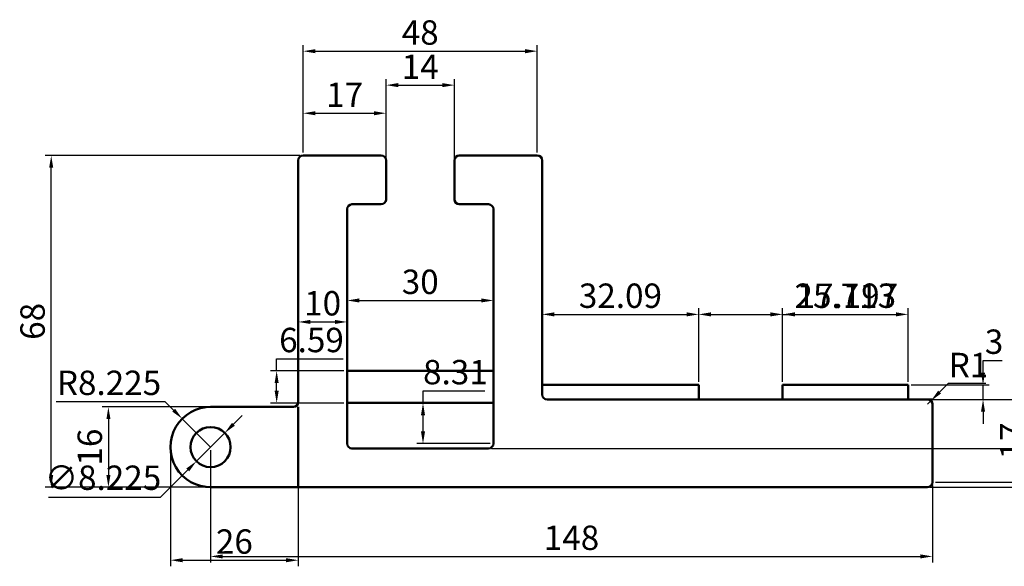
# Model space of a CAD drawing. Units: millimetres. Extents: x 2010 to 2347, y 1200 to 1429.
# Tile 2 of 3: x 2010 to 2212, y 1317 to 1429. Entities that reach past the tile are written whole.
import ezdxf

# ---------------------------------------------------------------- set-up
doc = ezdxf.new("R2010")
doc.units = ezdxf.units.MM
doc.layers.add('M-DIMS', color=2, linetype='Continuous', lineweight=25)
doc.layers.add('M-OUTL', color=7, linetype='Continuous', lineweight=50)
doc.styles.get("Standard").update_dxf_attribs({"font": 'arial.ttf'})
doc.dimstyles.new('ISO-25', dxfattribs={"dimtxt": 5, "dimasz": 2.5, "dimexe": 1.25, "dimexo": 0.625, "dimtad": 1, "dimtoh": 1, "dimdec": 0, "dimtxsty": 'Standard', "dimcen": 2.5, "dimadec": 0, "dimazin": 0, "dimtfac": 1, "dimtdec": 0, "dimtmove": 0, "dimatfit": 3, "dimfxl": 1, "dimarcsym": 0})

# ---------------------------------------------------------------- blocks, each defined once
blk = doc.blocks.new('*D1')
at = {"layer": 'Defpoints', "color": 0, "transparency": 16777216}
for p in [(2049.6, 1341.27), (2197.57, 1334.05), (2197.57, 1318.86)]:
    blk.add_point(p, dxfattribs=at)
at = {"layer": 'M-DIMS', "color": 0, "lineweight": -2, "transparency": 16777216}
for p, q in [((2049.6, 1340.65), (2049.6, 1317.61)), ((2197.57, 1333.42), (2197.57, 1317.61)), ((2052.1, 1318.86), (2195.07, 1318.86))]:
    blk.add_line(p, q, dxfattribs=at)
at = {"layer": 'M-DIMS', "color": 0, "transparency": 16777216}
for points in [[(2052.1, 1319.27), (2052.1, 1318.44), (2049.6, 1318.86)], [(2195.07, 1319.27), (2195.07, 1318.44), (2197.57, 1318.86)]]:
    blk.add_solid(points, dxfattribs=at)
at = {"layer": 'M-DIMS', "color": 0, "transparency": 16777216, "insert": (2123.58, 1322.03), "char_height": 5, "attachment_point": 5}
blk.add_mtext('148', dxfattribs=at)
blk = doc.blocks.new('*D2')
at = {"layer": 'Defpoints', "color": 0, "transparency": 16777216}
for p in [(2196.57, 1351.05), (2217.71, 1351.05), (2197.57, 1334.05)]:
    blk.add_point(p, dxfattribs=at)
at = {"layer": 'M-DIMS', "color": 0, "lineweight": -2, "transparency": 16777216}
for p, q in [((2197.19, 1351.05), (2218.96, 1351.05)), ((2217.71, 1336.55), (2217.71, 1348.55)), ((2198.19, 1334.05), (2218.96, 1334.05))]:
    blk.add_line(p, q, dxfattribs=at)
at = {"layer": 'M-DIMS', "color": 0, "transparency": 16777216}
for points in [[(2217.3, 1348.55), (2218.13, 1348.55), (2217.71, 1351.05)], [(2217.3, 1336.55), (2218.13, 1336.55), (2217.71, 1334.05)]]:
    blk.add_solid(points, dxfattribs=at)
at = {"layer": 'M-DIMS', "color": 0, "transparency": 16777216, "insert": (2214.58, 1342.55), "char_height": 5, "attachment_point": 5, "rotation": 90}
blk.add_mtext('17', dxfattribs=at)
blk = doc.blocks.new('*D3')
at = {"layer": 'Defpoints', "color": 0, "transparency": 16777216}
for p in [(2192.57, 1354.05), (2207.94, 1354.05), (2196.57, 1351.05)]:
    blk.add_point(p, dxfattribs=at)
at = {"layer": 'M-DIMS', "color": 0, "lineweight": -2, "transparency": 16777216}
for p, q in [((2207.94, 1356.55), (2207.94, 1359.05)), ((2207.94, 1359.05), (2211.84, 1359.05)), ((2193.19, 1354.05), (2209.19, 1354.05)), ((2207.94, 1351.05), (2207.94, 1354.05)), ((2197.19, 1351.05), (2209.19, 1351.05)), ((2207.94, 1348.55), (2207.94, 1346.05))]:
    blk.add_line(p, q, dxfattribs=at)
at = {"layer": 'M-DIMS', "color": 0, "transparency": 16777216}
for points in [[(2207.52, 1356.55), (2208.35, 1356.55), (2207.94, 1354.05)], [(2207.52, 1348.55), (2208.35, 1348.55), (2207.94, 1351.05)]]:
    blk.add_solid(points, dxfattribs=at)
at = {"layer": 'M-DIMS', "color": 0, "transparency": 16777216, "insert": (2210.2, 1362.23), "char_height": 5, "attachment_point": 5}
blk.add_mtext('3', dxfattribs=at)
blk = doc.blocks.new('*D4')
at = {"layer": 'Defpoints', "color": 0, "transparency": 16777216}
for p in [(2041.37, 1341.27), (2067.57, 1341.27), (2067.57, 1318.08)]:
    blk.add_point(p, dxfattribs=at)
at = {"layer": 'M-DIMS', "color": 0, "lineweight": -2, "transparency": 16777216}
for p, q in [((2041.37, 1340.65), (2041.37, 1316.83)), ((2067.57, 1340.65), (2067.57, 1316.83)), ((2043.87, 1318.08), (2065.07, 1318.08))]:
    blk.add_line(p, q, dxfattribs=at)
at = {"layer": 'M-DIMS', "color": 0, "transparency": 16777216}
for points in [[(2043.87, 1318.5), (2043.87, 1317.66), (2041.37, 1318.08)], [(2065.07, 1318.5), (2065.07, 1317.66), (2067.57, 1318.08)]]:
    blk.add_solid(points, dxfattribs=at)
at = {"layer": 'M-DIMS', "color": 0, "transparency": 16777216, "insert": (2054.47, 1321.26), "char_height": 5, "attachment_point": 5}
blk.add_mtext('26', dxfattribs=at)
blk = doc.blocks.new('*D5')
at = {"layer": 'Defpoints', "color": 0, "transparency": 16777216}
for p in [(2049.6, 1349.5), (2028.65, 1333.05), (2049.62, 1333.05)]:
    blk.add_point(p, dxfattribs=at)
at = {"layer": 'M-DIMS', "color": 0, "lineweight": -2, "transparency": 16777216}
for p, q in [((2048.97, 1349.5), (2027.4, 1349.5)), ((2028.65, 1347), (2028.65, 1335.55)), ((2049, 1333.05), (2027.4, 1333.05))]:
    blk.add_line(p, q, dxfattribs=at)
at = {"layer": 'M-DIMS', "color": 0, "transparency": 16777216}
for points in [[(2028.24, 1347), (2029.07, 1347), (2028.65, 1349.5)], [(2028.24, 1335.55), (2029.07, 1335.55), (2028.65, 1333.05)]]:
    blk.add_solid(points, dxfattribs=at)
at = {"layer": 'M-DIMS', "color": 0, "transparency": 16777216, "insert": (2025.48, 1341.27), "char_height": 5, "attachment_point": 5, "rotation": 90}
blk.add_mtext('16', dxfattribs=at)
blk = doc.blocks.new('*D6')
at = {"layer": 'Defpoints', "color": 0, "transparency": 16777216}
for p in [(2067.57, 1375.27), (2077.57, 1366.93), (2077.57, 1366.03)]:
    blk.add_point(p, dxfattribs=at)
at = {"layer": 'M-DIMS', "color": 0, "lineweight": -2, "transparency": 16777216}
for p, q in [((2067.57, 1374.65), (2067.57, 1365.68)), ((2070.07, 1366.93), (2075.07, 1366.93)), ((2077.57, 1366.65), (2077.57, 1368.18))]:
    blk.add_line(p, q, dxfattribs=at)
at = {"layer": 'M-DIMS', "color": 0, "transparency": 16777216}
for points in [[(2070.07, 1367.35), (2070.07, 1366.51), (2067.57, 1366.93)], [(2075.07, 1367.35), (2075.07, 1366.51), (2077.57, 1366.93)]]:
    blk.add_solid(points, dxfattribs=at)
at = {"layer": 'M-DIMS', "color": 0, "transparency": 16777216, "insert": (2072.57, 1370.11), "char_height": 5, "attachment_point": 5}
blk.add_mtext('10', dxfattribs=at)
blk = doc.blocks.new('*D7')
at = {"layer": 'Defpoints', "color": 0, "transparency": 16777216}
for p in [(2085.57, 1409.72), (2068.57, 1401.05), (2085.57, 1400.05)]:
    blk.add_point(p, dxfattribs=at)
at = {"layer": 'M-DIMS', "color": 0, "lineweight": -2, "transparency": 16777216}
for p, q in [((2068.57, 1401.67), (2068.57, 1410.97)), ((2085.57, 1400.67), (2085.57, 1410.97)), ((2071.07, 1409.72), (2083.07, 1409.72))]:
    blk.add_line(p, q, dxfattribs=at)
at = {"layer": 'M-DIMS', "color": 0, "transparency": 16777216}
for points in [[(2071.07, 1410.13), (2071.07, 1409.3), (2068.57, 1409.72)], [(2083.07, 1410.13), (2083.07, 1409.3), (2085.57, 1409.72)]]:
    blk.add_solid(points, dxfattribs=at)
at = {"layer": 'M-DIMS', "color": 0, "transparency": 16777216, "insert": (2077.07, 1412.85), "char_height": 5, "attachment_point": 5}
blk.add_mtext('17', dxfattribs=at)
blk = doc.blocks.new('*D8')
at = {"layer": 'Defpoints', "color": 0, "transparency": 16777216}
for p in [(2116.57, 1422.44), (2068.57, 1401.05), (2116.57, 1401.05)]:
    blk.add_point(p, dxfattribs=at)
at = {"layer": 'M-DIMS', "color": 0, "lineweight": -2, "transparency": 16777216}
for p, q in [((2068.57, 1401.67), (2068.57, 1423.69)), ((2116.57, 1401.67), (2116.57, 1423.69)), ((2071.07, 1422.44), (2114.07, 1422.44))]:
    blk.add_line(p, q, dxfattribs=at)
at = {"layer": 'M-DIMS', "color": 0, "transparency": 16777216}
for points in [[(2071.07, 1422.86), (2071.07, 1422.02), (2068.57, 1422.44)], [(2114.07, 1422.86), (2114.07, 1422.02), (2116.57, 1422.44)]]:
    blk.add_solid(points, dxfattribs=at)
at = {"layer": 'M-DIMS', "color": 0, "transparency": 16777216, "insert": (2092.57, 1425.62), "char_height": 5, "attachment_point": 5}
blk.add_mtext('48', dxfattribs=at)
blk = doc.blocks.new('*D25')
at = {"layer": 'Defpoints', "color": 0, "transparency": 16777216}
for p in [(2016.93, 1401.05), (2068.57, 1401.05), (2049.62, 1333.05)]:
    blk.add_point(p, dxfattribs=at)
at = {"layer": 'M-DIMS', "color": 0, "lineweight": -2, "transparency": 16777216}
for p, q in [((2067.94, 1401.05), (2015.68, 1401.05)), ((2016.93, 1335.55), (2016.93, 1398.55)), ((2049, 1333.05), (2015.68, 1333.05))]:
    blk.add_line(p, q, dxfattribs=at)
at = {"layer": 'M-DIMS', "color": 0, "transparency": 16777216}
for points in [[(2016.51, 1398.55), (2017.34, 1398.55), (2016.93, 1401.05)], [(2016.51, 1335.55), (2017.34, 1335.55), (2016.93, 1333.05)]]:
    blk.add_solid(points, dxfattribs=at)
at = {"layer": 'M-DIMS', "color": 0, "transparency": 16777216, "insert": (2013.75, 1367.05), "char_height": 5, "attachment_point": 5, "rotation": 90}
blk.add_mtext('68', dxfattribs=at)
blk = doc.blocks.new('*D32')
at = {"layer": 'Defpoints', "color": 0, "transparency": 16777216}
for p in [(2099.57, 1415.48), (2085.57, 1400.05), (2099.57, 1400.05)]:
    blk.add_point(p, dxfattribs=at)
at = {"layer": 'M-DIMS', "color": 0, "lineweight": -2, "transparency": 16777216}
for p, q in [((2085.57, 1400.67), (2085.57, 1416.73)), ((2088.07, 1415.48), (2097.07, 1415.48)), ((2099.57, 1400.67), (2099.57, 1416.73))]:
    blk.add_line(p, q, dxfattribs=at)
at = {"layer": 'M-DIMS', "color": 0, "transparency": 16777216}
for points in [[(2088.07, 1415.9), (2088.07, 1415.06), (2085.57, 1415.48)], [(2097.07, 1415.9), (2097.07, 1415.06), (2099.57, 1415.48)]]:
    blk.add_solid(points, dxfattribs=at)
at = {"layer": 'M-DIMS', "color": 0, "transparency": 16777216, "insert": (2092.57, 1418.61), "char_height": 5, "attachment_point": 5}
blk.add_mtext('14', dxfattribs=at)
blk = doc.blocks.new('*D36')
at = {"layer": 'Defpoints', "color": 0, "transparency": 16777216}
for p in [(2106.57, 1341), (2329.76, 1341), (2196.57, 1333.05)]:
    blk.add_point(p, dxfattribs=at)
at = {"layer": 'M-DIMS', "color": 0, "lineweight": -2, "transparency": 16777216}
for p, q in [((2329.76, 1341), (2329.76, 1343.5)), ((2329.76, 1343.5), (2347.26, 1343.5)), ((2107.19, 1341), (2331.01, 1341)), ((2329.76, 1335.55), (2329.76, 1338.5)), ((2197.19, 1333.05), (2331.01, 1333.05))]:
    blk.add_line(p, q, dxfattribs=at)
at = {"layer": 'M-DIMS', "color": 0, "transparency": 16777216}
for points in [[(2329.35, 1338.5), (2330.18, 1338.5), (2329.76, 1341)], [(2329.35, 1335.55), (2330.18, 1335.55), (2329.76, 1333.05)]]:
    blk.add_solid(points, dxfattribs=at)
at = {"layer": 'M-DIMS', "color": 0, "transparency": 16777216, "insert": (2338.82, 1346.68), "char_height": 5, "attachment_point": 5}
blk.add_mtext('7.955', dxfattribs=at)
blk = doc.blocks.new('*D37')
at = {"layer": 'Defpoints', "color": 0, "transparency": 16777216}
for p in [(2063.14, 1356.9), (2077.57, 1356.9), (2077.57, 1350.31)]:
    blk.add_point(p, dxfattribs=at)
at = {"layer": 'M-DIMS', "color": 0, "lineweight": -2, "transparency": 16777216}
for p, q in [((2063.14, 1356.9), (2063.14, 1359.4)), ((2063.14, 1359.4), (2076.79, 1359.4)), ((2076.94, 1356.9), (2061.89, 1356.9)), ((2063.14, 1352.81), (2063.14, 1354.4)), ((2076.94, 1350.31), (2061.89, 1350.31))]:
    blk.add_line(p, q, dxfattribs=at)
at = {"layer": 'M-DIMS', "color": 0, "transparency": 16777216}
for points in [[(2062.72, 1354.4), (2063.56, 1354.4), (2063.14, 1356.9)], [(2062.72, 1352.81), (2063.56, 1352.81), (2063.14, 1350.31)]]:
    blk.add_solid(points, dxfattribs=at)
at = {"layer": 'M-DIMS', "color": 0, "transparency": 16777216, "insert": (2070.28, 1362.58), "char_height": 5, "attachment_point": 5}
blk.add_mtext('6.59', dxfattribs=at)
blk = doc.blocks.new('*D38')
at = {"layer": 'Defpoints', "color": 0, "transparency": 16777216}
for p in [(2149.66, 1368.48), (2117.57, 1354.05), (2149.66, 1354.05)]:
    blk.add_point(p, dxfattribs=at)
at = {"layer": 'M-DIMS', "color": 0, "lineweight": -2, "transparency": 16777216}
for p, q in [((2117.57, 1354.67), (2117.57, 1369.73)), ((2120.07, 1368.48), (2147.16, 1368.48)), ((2149.66, 1354.67), (2149.66, 1369.73))]:
    blk.add_line(p, q, dxfattribs=at)
at = {"layer": 'M-DIMS', "color": 0, "transparency": 16777216}
for points in [[(2120.07, 1368.9), (2120.07, 1368.06), (2117.57, 1368.48)], [(2147.16, 1368.9), (2147.16, 1368.06), (2149.66, 1368.48)]]:
    blk.add_solid(points, dxfattribs=at)
at = {"layer": 'M-DIMS', "color": 0, "transparency": 16777216, "insert": (2133.61, 1371.66), "char_height": 5, "attachment_point": 5}
blk.add_mtext('32.09', dxfattribs=at)
blk = doc.blocks.new('*D39')
at = {"layer": 'Defpoints', "color": 0, "transparency": 16777216}
for p in [(2166.86, 1368.48), (2149.66, 1354.05), (2166.86, 1354.05)]:
    blk.add_point(p, dxfattribs=at)
at = {"layer": 'M-DIMS', "color": 0, "lineweight": -2, "transparency": 16777216}
for p, q in [((2149.66, 1354.67), (2149.66, 1369.73)), ((2152.16, 1368.48), (2164.36, 1368.48)), ((2166.86, 1354.67), (2166.86, 1369.73)), ((2166.86, 1368.48), (2190.89, 1368.48))]:
    blk.add_line(p, q, dxfattribs=at)
at = {"layer": 'M-DIMS', "color": 0, "transparency": 16777216}
for points in [[(2152.16, 1368.9), (2152.16, 1368.06), (2149.66, 1368.48)], [(2164.36, 1368.9), (2164.36, 1368.06), (2166.86, 1368.48)]]:
    blk.add_solid(points, dxfattribs=at)
at = {"layer": 'M-DIMS', "color": 0, "transparency": 16777216, "insert": (2180.12, 1371.66), "char_height": 5, "attachment_point": 5}
blk.add_mtext('17.197', dxfattribs=at)
blk = doc.blocks.new('*D40')
at = {"layer": 'Defpoints', "color": 0, "transparency": 16777216}
for p in [(2192.57, 1368.48), (2166.86, 1354.05), (2192.57, 1354.05)]:
    blk.add_point(p, dxfattribs=at)
at = {"layer": 'M-DIMS', "color": 0, "lineweight": -2, "transparency": 16777216}
for p, q in [((2166.86, 1354.67), (2166.86, 1369.73)), ((2169.36, 1368.48), (2190.07, 1368.48)), ((2192.57, 1354.67), (2192.57, 1369.73))]:
    blk.add_line(p, q, dxfattribs=at)
at = {"layer": 'M-DIMS', "color": 0, "transparency": 16777216}
for points in [[(2169.36, 1368.9), (2169.36, 1368.06), (2166.86, 1368.48)], [(2190.07, 1368.9), (2190.07, 1368.06), (2192.57, 1368.48)]]:
    blk.add_solid(points, dxfattribs=at)
at = {"layer": 'M-DIMS', "color": 0, "transparency": 16777216, "insert": (2179.71, 1371.66), "char_height": 5, "attachment_point": 5}
blk.add_mtext('25.713', dxfattribs=at)
blk = doc.blocks.new('*D41')
at = {"layer": 'Defpoints', "color": 0, "transparency": 16777216}
for p in [(2093.14, 1350.31), (2107.57, 1350.31), (2107.57, 1342)]:
    blk.add_point(p, dxfattribs=at)
at = {"layer": 'M-DIMS', "color": 0, "lineweight": -2, "transparency": 16777216}
for p, q in [((2093.14, 1350.31), (2093.14, 1352.81)), ((2093.14, 1352.81), (2105.79, 1352.81)), ((2106.94, 1350.31), (2091.89, 1350.31)), ((2093.14, 1344.5), (2093.14, 1347.81)), ((2106.94, 1342), (2091.89, 1342))]:
    blk.add_line(p, q, dxfattribs=at)
at = {"layer": 'M-DIMS', "color": 0, "transparency": 16777216}
for points in [[(2092.72, 1347.81), (2093.56, 1347.81), (2093.14, 1350.31)], [(2092.72, 1344.5), (2093.56, 1344.5), (2093.14, 1342)]]:
    blk.add_solid(points, dxfattribs=at)
at = {"layer": 'M-DIMS', "color": 0, "transparency": 16777216, "insert": (2099.78, 1355.99), "char_height": 5, "attachment_point": 5}
blk.add_mtext('8.31', dxfattribs=at)
blk = doc.blocks.new('*D44')
at = {"layer": 'Defpoints', "color": 0, "transparency": 16777216}
for p in [(2107.57, 1371.33), (2077.57, 1356.9), (2107.57, 1356.9)]:
    blk.add_point(p, dxfattribs=at)
at = {"layer": 'M-DIMS', "color": 0, "lineweight": -2, "transparency": 16777216}
for p, q in [((2077.57, 1357.53), (2077.57, 1372.58)), ((2107.57, 1357.53), (2107.57, 1372.58)), ((2080.07, 1371.33), (2105.07, 1371.33))]:
    blk.add_line(p, q, dxfattribs=at)
at = {"layer": 'M-DIMS', "color": 0, "transparency": 16777216}
for points in [[(2080.07, 1371.75), (2080.07, 1370.92), (2077.57, 1371.33)], [(2105.07, 1371.75), (2105.07, 1370.92), (2107.57, 1371.33)]]:
    blk.add_solid(points, dxfattribs=at)
at = {"layer": 'M-DIMS', "color": 0, "transparency": 16777216, "insert": (2092.57, 1374.51), "char_height": 5, "attachment_point": 5}
blk.add_mtext('30', dxfattribs=at)
blk = doc.blocks.new('*D51')
at = {"layer": 'Defpoints', "color": 0, "transparency": 16777216}
for p in [(2043.78, 1347.09), (2049.6, 1341.27)]:
    blk.add_point(p, dxfattribs=at)
at = {"layer": 'M-DIMS', "color": 0, "lineweight": -2, "transparency": 16777216}
for p, q in [((2017.92, 1350.63), (2040.24, 1350.63)), ((2040.24, 1350.63), (2042.01, 1348.86)), ((2049.6, 1341.27), (2043.78, 1347.09))]:
    blk.add_line(p, q, dxfattribs=at)
at = {"layer": 'M-DIMS', "color": 0, "transparency": 16777216}
blk.add_solid([(2042.31, 1349.15), (2041.72, 1348.56), (2043.78, 1347.09)], dxfattribs=at)
at = {"layer": 'M-DIMS', "color": 0, "transparency": 16777216, "insert": (2028.77, 1353.8), "char_height": 5, "attachment_point": 5}
blk.add_mtext('R8.225', dxfattribs=at)
blk = doc.blocks.new('*D52')
at = {"layer": 'Defpoints', "color": 0, "transparency": 16777216}
for p in [(2052.5, 1344.18), (2046.69, 1338.37)]:
    blk.add_point(p, dxfattribs=at)
at = {"layer": 'M-DIMS', "color": 0, "lineweight": -2, "transparency": 16777216}
for p, q in [((2054.27, 1345.95), (2056.04, 1347.72)), ((2052.5, 1344.18), (2046.69, 1338.37)), ((2039.34, 1331.03), (2044.92, 1336.6)), ((2016.37, 1331.03), (2039.34, 1331.03))]:
    blk.add_line(p, q, dxfattribs=at)
at = {"layer": 'M-DIMS', "color": 0, "transparency": 16777216}
for points in [[(2053.98, 1346.24), (2054.57, 1345.65), (2052.5, 1344.18)], [(2044.62, 1336.89), (2045.21, 1336.3), (2046.69, 1338.37)]]:
    blk.add_solid(points, dxfattribs=at)
at = {"layer": 'M-DIMS', "color": 0, "transparency": 16777216, "insert": (2027.54, 1334.34), "char_height": 5, "attachment_point": 5}
blk.add_mtext('∅8.225', dxfattribs=at)
blk = doc.blocks.new('*D53')
at = {"layer": 'Defpoints', "color": 0, "transparency": 16777216}
for p in [(2197.27, 1350.76), (2196.57, 1350.05)]:
    blk.add_point(p, dxfattribs=at)
at = {"layer": 'M-DIMS', "color": 0, "lineweight": -2, "transparency": 16777216}
for p, q in [((2200.78, 1354.32), (2199.03, 1352.54)), ((2208.51, 1354.32), (2200.78, 1354.32)), ((2196.57, 1350.05), (2197.27, 1350.76))]:
    blk.add_line(p, q, dxfattribs=at)
at = {"layer": 'M-DIMS', "color": 0, "transparency": 16777216}
blk.add_solid([(2198.73, 1352.83), (2199.32, 1352.25), (2197.27, 1350.76)], dxfattribs=at)
at = {"layer": 'M-DIMS', "color": 0, "transparency": 16777216, "insert": (2204.96, 1357.45), "char_height": 5, "attachment_point": 5}
blk.add_mtext('R1', dxfattribs=at)

msp = doc.modelspace()

# ---------------------------------------------------------------- linework, layer by layer
at = {"layer": 'M-OUTL'}
for p, q in [((2068.5687, 1401.0495), (2084.5687, 1401.0495)), ((2116.5687, 1401.0495), (2100.5687, 1401.0495)), ((2067.5687, 1400.0495), (2067.5687, 1350.4977)), ((2085.5687, 1400.0495), (2085.5687, 1392.0495)), ((2099.5687, 1400.0495), (2099.5687, 1392.0495)), ((2117.5687, 1352.0495), (2117.5687, 1400.0495)), ((2084.5687, 1391.0495), (2078.5687, 1391.0495)), ((2100.5687, 1391.0495), (2106.5687, 1391.0495)), ((2077.5687, 1390.0495), (2077.5687, 1342.0047)), ((2107.5687, 1390.0495), (2107.5687, 1342.0047)), ((2077.5687, 1356.9049), (2107.5687, 1356.9049)), ((2117.5687, 1352.0495), (2117.5687, 1354.0495)), ((2117.5687, 1354.0495), (2149.6588, 1354.0495)), ((2149.6588, 1354.0495), (2149.6588, 1351.0495)), ((2192.5687, 1354.0495), (2166.8556, 1354.0495)), ((2166.8556, 1354.0495), (2166.8556, 1351.0495)), ((2192.5687, 1351.0495), (2192.5687, 1354.0495)), ((2077.5687, 1350.3146), (2107.5687, 1350.3146)), ((2197.5687, 1351.0495), (2118.5687, 1351.0495)), ((2196.5687, 1351.0495), (2192.5687, 1351.0495)), ((2066.5687, 1349.4977), (2049.5687, 1349.4977)), ((2067.5687, 1349.4977), (2067.5687, 1333.0495)), ((2197.5687, 1334.0495), (2197.5687, 1350.0495)), ((2078.5687, 1341.0047), (2105.1045, 1341.0047)), ((2105.1045, 1341.0047), (2106.5687, 1341.0047)), ((2057.5687, 1333.0495), (2049.622, 1333.0495)), ((2057.5687, 1333.0495), (2196.5687, 1333.0495))]:
    msp.add_line(p, q, dxfattribs=at)
msp.add_circle((2049.5953, 1341.2736), 4.1125, dxfattribs=at)
for centre, radius, start, end in [((2068.5687, 1400.0495), 1, 90, 180), ((2084.5687, 1400.0495), 1, 0, 90), ((2100.5687, 1400.0495), 1, 90, 180), ((2116.5687, 1400.0495), 1, 0, 90), ((2078.5687, 1390.0495), 1, 90, 180), ((2084.5687, 1392.0495), 1, 270, 0), ((2100.5687, 1392.0495), 1, 180, 270), ((2106.5687, 1390.0495), 1, 0, 90), ((2066.5687, 1350.4977), 1, 270, 0), ((2118.5687, 1352.0495), 1, 180, 270), ((2196.5687, 1350.0495), 1, 0, 90), ((2049.5953, 1341.2736), 8.225, 89.146623, 270.853377), ((2078.5687, 1342.0047), 1, 180, 270), ((2106.5687, 1342.0047), 1, 270, 0), ((2196.5687, 1334.0495), 1, 270, 0)]:
    msp.add_arc(centre, radius, start, end, dxfattribs=at)

# ---------------------------------------------------------------- dimensions: what is measured, and where the dimension line sits
at = {"layer": 'M-DIMS'}
for base, p1, p2, override, picture, middle in [((2116.5687, 1422.4386), (2068.5687, 1401.0495), (2116.5687, 1401.0495), {"dimclrd": 0, "dimclre": 0, "dimclrt": 0}, '*D8', (2092.5687, 1425.6165)), ((2099.5687, 1415.4795), (2085.5687, 1400.0495), (2099.5687, 1400.0495), {"dimdec": 0, "dimlfac": 1, "dimrnd": 0, "dimzin": 0, "dimdsep": 46, "dimlunit": 2}, '*D32', (2092.5687, 1418.6148)), ((2085.5687, 1409.7167), (2068.5687, 1401.0495), (2085.5687, 1400.0495), {"dimclrd": 0, "dimclre": 0, "dimclrt": 0}, '*D7', (2077.0687, 1412.8519)), ((2107.5687, 1371.3349), (2077.5687, 1356.9049), (2107.5687, 1356.9049), {"dimdec": 0, "dimlfac": 1, "dimrnd": 0, "dimzin": 0, "dimdsep": 46, "dimlunit": 2}, '*D44', (2092.5687, 1374.5145)), ((2077.5687, 1366.9311), (2067.5687, 1375.2736), (2077.5687, 1366.0271), {"dimclrd": 0, "dimclre": 0, "dimclrt": 0}, '*D6', (2072.5687, 1370.109)), ((2149.6588, 1368.4795), (2117.5687, 1354.0495), (2149.6588, 1354.0495), {"dimdec": 2, "dimlfac": 1, "dimrnd": 0, "dimzin": 0, "dimdsep": 46, "dimlunit": 2}, '*D38', (2133.6137, 1371.6591)), ((2166.8556, 1368.4795), (2149.6588, 1354.0495), (2166.8556, 1354.0495), {"dimdec": 3, "dimlfac": 1, "dimrnd": 0, "dimzin": 0, "dimdsep": 46, "dimlunit": 2}, '*D39', (2180.1238, 1371.6574)), ((2192.5687, 1368.4795), (2166.8556, 1354.0495), (2192.5687, 1354.0495), {"dimdec": 3, "dimlfac": 1, "dimrnd": 0, "dimzin": 0, "dimdsep": 46, "dimlunit": 2}, '*D40', (2179.7121, 1371.6591)), ((2067.5687, 1318.0789), (2041.3703, 1341.2736), (2067.5687, 1341.2736), {"dimclrd": 0, "dimclre": 0, "dimclrt": 0}, '*D4', (2054.4695, 1321.2568)), ((2197.5687, 1318.8555), (2049.5953, 1341.2736), (2197.5687, 1334.0495), {"dimclrd": 0, "dimclre": 0, "dimclrt": 0}, '*D1', (2123.582, 1322.0334))]:
    dim = msp.add_linear_dim(base=base, p1=p1, p2=p2, dimstyle='ISO-25', override=override, dxfattribs=at)
    dim.commit()
    dim.dimension.update_dxf_attribs({"geometry": picture, "text_midpoint": middle})
for base, p1, p2, override, picture, middle in [((2016.9251, 1401.0495), (2049.622, 1333.0495), (2068.5687, 1401.0495), {"dimdec": 0, "dimlfac": 1, "dimrnd": 0, "dimzin": 0, "dimdsep": 46, "dimlunit": 2}, '*D25', (2013.7472, 1367.0495)), ((2063.1387, 1356.9049), (2077.5687, 1350.3146), (2077.5687, 1356.9049), {"dimdec": 2, "dimlfac": 1, "dimrnd": 0, "dimzin": 0, "dimdsep": 46, "dimlunit": 2}, '*D37', (2070.2763, 1362.5827)), ((2207.9365, 1354.0495), (2196.5687, 1351.0495), (2192.5687, 1354.0495), {"dimclrd": 0, "dimclre": 0, "dimclrt": 0}, '*D3', (2210.1986, 1362.2291)), ((2093.1387, 1350.3146), (2107.5687, 1342.0047), (2107.5687, 1350.3146), {"dimdec": 2, "dimlfac": 1, "dimrnd": 0, "dimzin": 0, "dimdsep": 46, "dimlunit": 2}, '*D41', (2099.7784, 1355.9942)), ((2217.714, 1351.0495), (2197.5687, 1334.0495), (2196.5687, 1351.0495), {"dimclrd": 0, "dimclre": 0, "dimclrt": 0}, '*D2', (2214.5787, 1342.5495)), ((2028.6533, 1333.0495), (2049.5953, 1349.4986), (2049.622, 1333.0495), {"dimclrd": 0, "dimclre": 0, "dimclrt": 0}, '*D5', (2025.4755, 1341.2741)), ((2329.7618, 1341.0047), (2196.5687, 1333.0495), (2106.5687, 1341.0047), {"dimdec": 3, "dimlfac": 1, "dimrnd": 0, "dimzin": 0, "dimdsep": 46, "dimlunit": 2}, '*D36', (2338.8213, 1346.6825))]:
    dim = msp.add_linear_dim(base=base, p1=p1, p2=p2, angle=90, dimstyle='ISO-25', override=override, dxfattribs=at)
    dim.commit()
    dim.dimension.update_dxf_attribs({"geometry": picture, "text_midpoint": middle})
for center, mpoint, override, picture, middle in [((2196.5687, 1350.0495), (2197.2712, 1350.7612), {"dimdec": 0, "dimlfac": 1, "dimrnd": 0, "dimzin": 0, "dimdsep": 46, "dimlunit": 2}, '*D53', (2204.9575, 1357.4549)), ((2049.5953, 1341.2736), (2043.7799, 1347.0901), {"dimdec": 3, "dimlfac": 1, "dimrnd": 0, "dimzin": 0, "dimdsep": 46, "dimlunit": 2}, '*D51', (2028.7721, 1353.8038))]:
    dim = msp.add_radius_dim(center=center, mpoint=mpoint, dimstyle='ISO-25', override=override, dxfattribs=at)
    dim.commit()
    dim.dimension.update_dxf_attribs({"geometry": picture, "text_midpoint": middle})
dim = msp.add_diameter_dim_2p(p1=(2052.5042, 1344.1807), p2=(2046.6865, 1338.3665), dimstyle='ISO-25', override={"dimdec": 3, "dimlfac": 1, "dimrnd": 0, "dimzin": 0, "dimdsep": 46, "dimlunit": 2}, dxfattribs=at)
dim.commit()
dim.dimension.update_dxf_attribs({"geometry": '*D52', "text_midpoint": (2027.5408, 1331.0251), "dimtype": 163})

doc.saveas('drawing.dxf')
